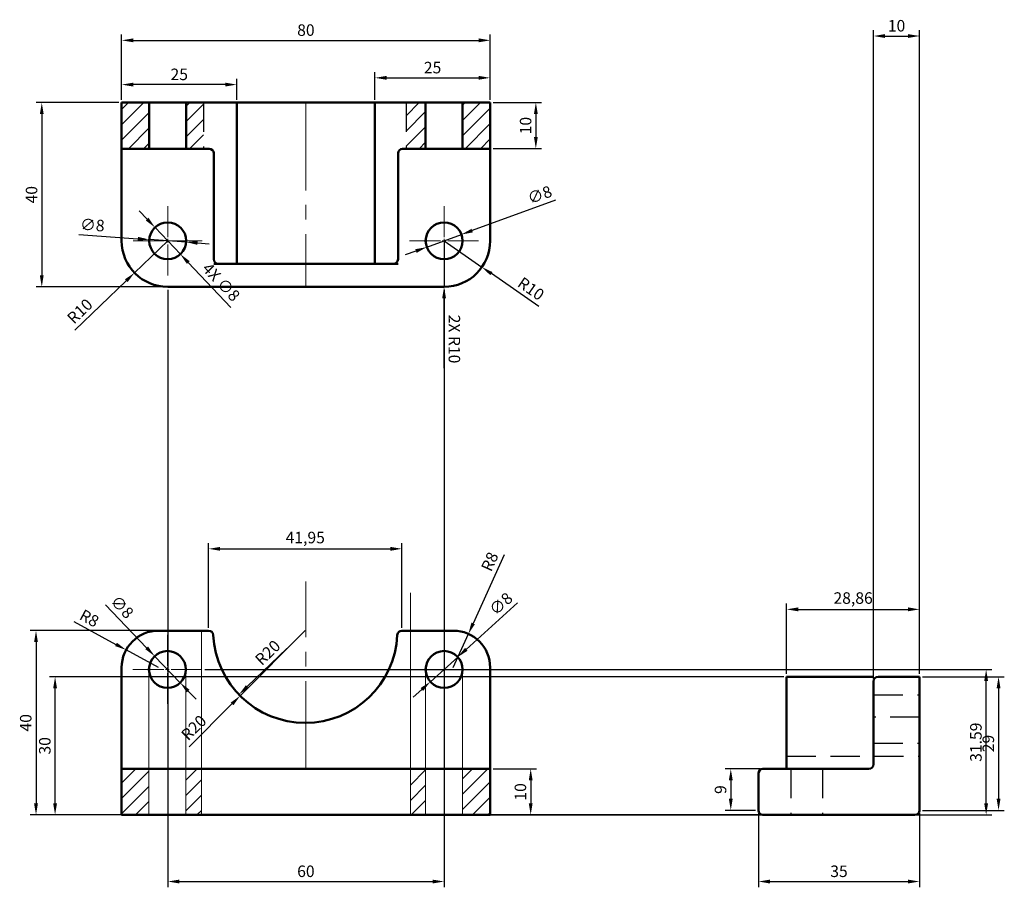
# Model space of a CAD drawing. Units: millimetres. Extents: x 1831 to 2045, y 920 to 1109.
import ezdxf

# ---------------------------------------------------------------- set-up
doc = ezdxf.new("R2010")
doc.units = ezdxf.units.MM
doc.linetypes.add('CENTER2', pattern=[28.575, 19.05, -3.175, 3.175, -3.175])
doc.linetypes.add('HIDDEN', pattern=[9.525, 6.35, -3.175])
for name, color, linetype, lineweight in [('M-CNTR', 4, 'CENTER2', 18), ('M-CONS', 8, 'Continuous', 13), ('M-DIMS', 2, 'Continuous', 25), ('M-HATC', 8, 'Continuous', 18), ('M-HIDN', 3, 'HIDDEN', 25), ('M-OUTL', 7, 'Continuous', 50)]:
    doc.layers.add(name, color=color, linetype=linetype, lineweight=lineweight)
doc.styles.get("Standard").update_dxf_attribs({"font": 'arial.ttf'})
doc.dimstyles.new('ISO-25', dxfattribs={"dimtxt": 2.5, "dimasz": 2.5, "dimexe": 1.25, "dimexo": 0.625, "dimtad": 1, "dimtxsty": 'Standard', "dimcen": 2.5, "dimadec": 0, "dimazin": 0, "dimtfac": 1, "dimtmove": 0, "dimatfit": 3, "dimfxl": 1, "dimarcsym": 0})

# ---------------------------------------------------------------- blocks, each defined once
blk = doc.blocks.new('*D1')
at = {"layer": 'Defpoints', "color": 0, "lineweight": 30, "transparency": 16777216}
for p in [(1914.1, 993.68), (1872.14, 975.92), (1914.1, 975.92)]:
    blk.add_point(p, dxfattribs=at)
at = {"layer": 'M-DIMS', "color": 0, "lineweight": -2, "transparency": 16777216}
for p, q in [((1872.14, 976.54), (1872.14, 994.93)), ((1914.1, 976.54), (1914.1, 994.93)), ((1874.64, 993.68), (1911.6, 993.68))]:
    blk.add_line(p, q, dxfattribs=at)
at = {"layer": 'M-DIMS', "color": 0, "lineweight": 30, "transparency": 16777216}
for points in [[(1874.64, 994.09), (1874.64, 993.26), (1872.14, 993.68)], [(1911.6, 994.09), (1911.6, 993.26), (1914.1, 993.68)]]:
    blk.add_solid(points, dxfattribs=at)
at = {"layer": 'M-DIMS', "color": 0, "transparency": 16777216, "insert": (1893.12, 995.8), "char_height": 2.5, "attachment_point": 5}
blk.add_mtext('41,95', dxfattribs=at)
blk = doc.blocks.new('*D2')
at = {"layer": 'Defpoints', "color": 0, "lineweight": 30, "transparency": 16777216}
for p in [(1933.26, 1104.04), (1853.26, 1090.53), (1933.26, 1090.53)]:
    blk.add_point(p, dxfattribs=at)
at = {"layer": 'M-DIMS', "color": 0, "lineweight": -2, "transparency": 16777216}
for p, q in [((1853.26, 1091.15), (1853.26, 1105.29)), ((1933.26, 1091.15), (1933.26, 1105.29)), ((1855.76, 1104.04), (1930.76, 1104.04))]:
    blk.add_line(p, q, dxfattribs=at)
at = {"layer": 'M-DIMS', "color": 0, "lineweight": 30, "transparency": 16777216}
for points in [[(1855.76, 1104.46), (1855.76, 1103.62), (1853.26, 1104.04)], [(1930.76, 1104.46), (1930.76, 1103.62), (1933.26, 1104.04)]]:
    blk.add_solid(points, dxfattribs=at)
at = {"layer": 'M-DIMS', "color": 0, "transparency": 16777216, "insert": (1893.26, 1105.94), "char_height": 2.5, "attachment_point": 5}
blk.add_mtext('80', dxfattribs=at)
blk = doc.blocks.new('*D3')
at = {"layer": 'Defpoints', "color": 0, "lineweight": 30, "transparency": 16777216}
for p in [(1853.26, 1090.53), (1835.92, 1050.53), (1863.26, 1050.53)]:
    blk.add_point(p, dxfattribs=at)
at = {"layer": 'M-DIMS', "color": 0, "lineweight": -2, "transparency": 16777216}
for p, q in [((1852.63, 1090.53), (1834.67, 1090.53)), ((1835.92, 1088.03), (1835.92, 1053.03)), ((1862.63, 1050.53), (1834.67, 1050.53))]:
    blk.add_line(p, q, dxfattribs=at)
at = {"layer": 'M-DIMS', "color": 0, "lineweight": 30, "transparency": 16777216}
for points in [[(1835.5, 1088.03), (1836.33, 1088.03), (1835.92, 1090.53)], [(1835.5, 1053.03), (1836.33, 1053.03), (1835.92, 1050.53)]]:
    blk.add_solid(points, dxfattribs=at)
at = {"layer": 'M-DIMS', "color": 0, "transparency": 16777216, "insert": (1834.02, 1070.53), "char_height": 2.5, "attachment_point": 5, "rotation": 90}
blk.add_mtext('40', dxfattribs=at)
blk = doc.blocks.new('*U4')
at = {"layer": 'M-CNTR', "color": 0, "transparency": 16777216}
for p, q in [((0, 0.8), (0, 7.5)), ((-7.5, 0), (-0.8, 0)), ((0.8, 0), (7.5, 0)), ((0, -7.5), (0, -0.8))]:
    blk.add_line(p, q, dxfattribs=at)
at = {"layer": 'M-CNTR', "color": 0, "linetype": 'Continuous', "transparency": 16777216}
for p, q in [((-0.4, 0), (0.4, 0)), ((0, -0.4), (0, 0.4))]:
    blk.add_line(p, q, dxfattribs=at)
blk = doc.blocks.new('*U5')
at = {"layer": 'M-CNTR', "color": 0, "transparency": 16777216}
for p, q in [((0, 0.8), (0, 7.5)), ((-7.5, 0), (-0.8, 0)), ((0.8, 0), (7.5, 0)), ((0, -7.5), (0, -0.8))]:
    blk.add_line(p, q, dxfattribs=at)
at = {"layer": 'M-CNTR', "color": 0, "linetype": 'Continuous', "transparency": 16777216}
for p, q in [((-0.4, 0), (0.4, 0)), ((0, -0.4), (0, 0.4))]:
    blk.add_line(p, q, dxfattribs=at)
blk = doc.blocks.new('*U6')
at = {"layer": 'M-CNTR', "color": 0, "transparency": 16777216}
for p, q in [((0, 0.8), (0, 7.5)), ((-7.5, 0), (-0.8, 0)), ((0.8, 0), (7.5, 0)), ((0, -7.5), (0, -0.8))]:
    blk.add_line(p, q, dxfattribs=at)
at = {"layer": 'M-CNTR', "color": 0, "linetype": 'Continuous', "transparency": 16777216}
for p, q in [((-0.4, 0), (0.4, 0)), ((0, -0.4), (0, 0.4))]:
    blk.add_line(p, q, dxfattribs=at)
blk = doc.blocks.new('*U7')
at = {"layer": 'M-CNTR', "color": 0, "transparency": 16777216}
for p, q in [((0, 0.8), (0, 7.5)), ((-7.5, 0), (-0.8, 0)), ((0.8, 0), (7.5, 0)), ((0, -7.5), (0, -0.8))]:
    blk.add_line(p, q, dxfattribs=at)
at = {"layer": 'M-CNTR', "color": 0, "linetype": 'Continuous', "transparency": 16777216}
for p, q in [((-0.4, 0), (0.4, 0)), ((0, -0.4), (0, 0.4))]:
    blk.add_line(p, q, dxfattribs=at)
blk = doc.blocks.new('*D8')
at = {"layer": 'Defpoints', "color": 0, "lineweight": 30, "transparency": 16777216}
for p in [(1893.12, 975.92), (1878.71, 962.04)]:
    blk.add_point(p, dxfattribs=at)
at = {"layer": 'M-DIMS', "color": 0, "lineweight": -2, "transparency": 16777216}
blk.add_line((1889.11, 972.05), (1880.51, 963.78), dxfattribs=at)
at = {"layer": 'M-DIMS', "color": 0, "lineweight": 30, "transparency": 16777216}
blk.add_solid([(1880.23, 964.08), (1880.8, 963.48), (1878.71, 962.04)], dxfattribs=at)
at = {"layer": 'M-DIMS', "color": 0, "transparency": 16777216, "insert": (1885.19, 970.92), "char_height": 2.5, "attachment_point": 5, "rotation": 43.9159}
blk.add_mtext('R20', dxfattribs=at)
blk = doc.blocks.new('*D9')
at = {"layer": 'Defpoints', "color": 0, "lineweight": 30, "transparency": 16777216}
for p in [(1926.22, 970.19), (1920.29, 964.83)]:
    blk.add_point(p, dxfattribs=at)
at = {"layer": 'M-DIMS', "color": 0, "lineweight": -2, "transparency": 16777216}
for p, q in [((1939.21, 981.92), (1928.08, 971.86)), ((1920.29, 964.83), (1926.22, 970.19)), ((1918.43, 963.15), (1916.58, 961.48))]:
    blk.add_line(p, q, dxfattribs=at)
at = {"layer": 'M-DIMS', "color": 0, "lineweight": 30, "transparency": 16777216}
for points in [[(1927.8, 972.17), (1928.36, 971.56), (1926.22, 970.19)], [(1918.15, 963.46), (1918.71, 962.84), (1920.29, 964.83)]]:
    blk.add_solid(points, dxfattribs=at)
at = {"layer": 'M-DIMS', "color": 0, "transparency": 16777216, "insert": (1935.81, 981.5), "char_height": 2.5, "attachment_point": 5, "rotation": 42.0862}
blk.add_mtext('∅8', dxfattribs=at)
blk = doc.blocks.new('*D10')
at = {"layer": 'Defpoints', "color": 0, "lineweight": 30, "transparency": 16777216}
for p in [(1860.42, 970.39), (1865.96, 964.62)]:
    blk.add_point(p, dxfattribs=at)
at = {"layer": 'M-DIMS', "color": 0, "lineweight": -2, "transparency": 16777216}
for p, q in [((1849.76, 981.49), (1858.69, 972.2)), ((1865.96, 964.62), (1860.42, 970.39)), ((1867.69, 962.82), (1869.42, 961.02))]:
    blk.add_line(p, q, dxfattribs=at)
at = {"layer": 'M-DIMS', "color": 0, "lineweight": 30, "transparency": 16777216}
for points in [[(1858.99, 972.49), (1858.39, 971.91), (1860.42, 970.39)], [(1867.99, 963.11), (1867.39, 962.53), (1865.96, 964.62)]]:
    blk.add_solid(points, dxfattribs=at)
at = {"layer": 'M-DIMS', "color": 0, "transparency": 16777216, "insert": (1853.13, 980.83), "char_height": 2.5, "attachment_point": 5, "rotation": 313.8374}
blk.add_mtext('∅8', dxfattribs=at)
blk = doc.blocks.new('*D11')
at = {"layer": 'Defpoints', "color": 0, "lineweight": 30, "transparency": 16777216}
for p in [(1927.01, 1061.89), (1919.5, 1059.16)]:
    blk.add_point(p, dxfattribs=at)
at = {"layer": 'M-DIMS', "color": 0, "lineweight": -2, "transparency": 16777216}
for p, q in [((1947.43, 1069.32), (1929.36, 1062.75)), ((1919.5, 1059.16), (1927.01, 1061.89)), ((1917.15, 1058.31), (1914.8, 1057.45))]:
    blk.add_line(p, q, dxfattribs=at)
at = {"layer": 'M-DIMS', "color": 0, "lineweight": 30, "transparency": 16777216}
for points in [[(1929.22, 1063.14), (1929.51, 1062.36), (1927.01, 1061.89)], [(1917, 1058.7), (1917.29, 1057.91), (1919.5, 1059.16)]]:
    blk.add_solid(points, dxfattribs=at)
at = {"layer": 'M-DIMS', "color": 0, "transparency": 16777216, "insert": (1944.12, 1070.21), "char_height": 2.5, "attachment_point": 5, "rotation": 19.9841}
blk.add_mtext('∅8', dxfattribs=at)
blk = doc.blocks.new('*D12')
at = {"layer": 'Defpoints', "color": 0, "lineweight": 30, "transparency": 16777216}
for p in [(1859.27, 1060.8), (1867.25, 1060.25)]:
    blk.add_point(p, dxfattribs=at)
at = {"layer": 'M-DIMS', "color": 0, "lineweight": -2, "transparency": 16777216}
for p, q in [((1843.94, 1061.87), (1856.77, 1060.98)), ((1867.25, 1060.25), (1859.27, 1060.8)), ((1869.74, 1060.08), (1872.23, 1059.9))]:
    blk.add_line(p, q, dxfattribs=at)
at = {"layer": 'M-DIMS', "color": 0, "lineweight": 30, "transparency": 16777216}
for points in [[(1856.8, 1061.39), (1856.74, 1060.56), (1859.27, 1060.8)], [(1869.77, 1060.49), (1869.71, 1059.66), (1867.25, 1060.25)]]:
    blk.add_solid(points, dxfattribs=at)
at = {"layer": 'M-DIMS', "color": 0, "transparency": 16777216, "insert": (1846.88, 1063.64), "char_height": 2.5, "attachment_point": 5, "rotation": 356.0256}
blk.add_mtext('∅8', dxfattribs=at)
blk = doc.blocks.new('*D13')
at = {"layer": 'Defpoints', "color": 0, "lineweight": 30, "transparency": 16777216}
for p in [(1923.26, 1060.53), (1931.47, 1054.82)]:
    blk.add_point(p, dxfattribs=at)
at = {"layer": 'M-DIMS', "color": 0, "lineweight": -2, "transparency": 16777216}
for p, q in [((1923.26, 1060.53), (1931.47, 1054.82)), ((1943.83, 1046.24), (1933.52, 1053.4))]:
    blk.add_line(p, q, dxfattribs=at)
at = {"layer": 'M-DIMS', "color": 0, "lineweight": 30, "transparency": 16777216}
blk.add_solid([(1933.76, 1053.74), (1933.29, 1053.06), (1931.47, 1054.82)], dxfattribs=at)
at = {"layer": 'M-DIMS', "color": 0, "transparency": 16777216, "insert": (1941.95, 1049.86), "char_height": 2.5, "attachment_point": 5, "rotation": 325.2351}
blk.add_mtext('R10', dxfattribs=at)
blk = doc.blocks.new('*D14')
at = {"layer": 'Defpoints', "color": 0, "lineweight": 30, "transparency": 16777216}
for p in [(1863.26, 1060.53), (1856.05, 1053.59)]:
    blk.add_point(p, dxfattribs=at)
at = {"layer": 'M-DIMS', "color": 0, "lineweight": -2, "transparency": 16777216}
for p, q in [((1863.26, 1060.53), (1856.05, 1053.59)), ((1843.13, 1041.15), (1854.25, 1051.86))]:
    blk.add_line(p, q, dxfattribs=at)
at = {"layer": 'M-DIMS', "color": 0, "lineweight": 30, "transparency": 16777216}
blk.add_solid([(1853.96, 1052.16), (1854.54, 1051.56), (1856.05, 1053.59)], dxfattribs=at)
at = {"layer": 'M-DIMS', "color": 0, "transparency": 16777216, "insert": (1844.41, 1045.02), "char_height": 2.5, "attachment_point": 5, "rotation": 43.9113}
blk.add_mtext('R10', dxfattribs=at)
blk = doc.blocks.new('*D15')
at = {"layer": 'Defpoints', "color": 0, "lineweight": 30, "transparency": 16777216}
for p in [(1928.54, 975.21), (1925.26, 967.92)]:
    blk.add_point(p, dxfattribs=at)
at = {"layer": 'M-DIMS', "color": 0, "lineweight": -2, "transparency": 16777216}
for p, q in [((1936.28, 992.4), (1929.57, 977.49)), ((1925.26, 967.92), (1928.54, 975.21))]:
    blk.add_line(p, q, dxfattribs=at)
at = {"layer": 'M-DIMS', "color": 0, "lineweight": 30, "transparency": 16777216}
blk.add_solid([(1929.19, 977.66), (1929.95, 977.32), (1928.54, 975.21)], dxfattribs=at)
at = {"layer": 'M-DIMS', "color": 0, "transparency": 16777216, "insert": (1933.46, 990.77), "char_height": 2.5, "attachment_point": 5, "rotation": 65.7651}
blk.add_mtext('R8', dxfattribs=at)
blk = doc.blocks.new('*D16')
at = {"layer": 'Defpoints', "color": 0, "lineweight": 30, "transparency": 16777216}
for p in [(1854.23, 971.74), (1861.26, 967.92)]:
    blk.add_point(p, dxfattribs=at)
at = {"layer": 'M-DIMS', "color": 0, "lineweight": -2, "transparency": 16777216}
for p, q in [((1842.86, 977.93), (1852.03, 972.93)), ((1861.26, 967.92), (1854.23, 971.74))]:
    blk.add_line(p, q, dxfattribs=at)
at = {"layer": 'M-DIMS', "color": 0, "lineweight": 30, "transparency": 16777216}
blk.add_solid([(1852.23, 973.3), (1851.83, 972.57), (1854.23, 971.74)], dxfattribs=at)
at = {"layer": 'M-DIMS', "color": 0, "transparency": 16777216, "insert": (1846.09, 978.33), "char_height": 2.5, "attachment_point": 5, "rotation": 331.4476}
blk.add_mtext('R8', dxfattribs=at)
blk = doc.blocks.new('*D17')
at = {"layer": 'Defpoints', "color": 0, "lineweight": 30, "transparency": 16777216}
for p in [(1933.26, 945.92), (1933.26, 935.92), (1942.06, 935.92)]:
    blk.add_point(p, dxfattribs=at)
at = {"layer": 'M-DIMS', "color": 0, "lineweight": -2, "transparency": 16777216}
for p, q in [((1933.88, 945.92), (1943.31, 945.92)), ((1942.06, 943.42), (1942.06, 938.42)), ((1933.88, 935.92), (1943.31, 935.92))]:
    blk.add_line(p, q, dxfattribs=at)
at = {"layer": 'M-DIMS', "color": 0, "lineweight": 30, "transparency": 16777216}
for points in [[(1941.65, 943.42), (1942.48, 943.42), (1942.06, 945.92)], [(1941.65, 938.42), (1942.48, 938.42), (1942.06, 935.92)]]:
    blk.add_solid(points, dxfattribs=at)
at = {"layer": 'M-DIMS', "color": 0, "transparency": 16777216, "insert": (1940.16, 940.92), "char_height": 2.5, "attachment_point": 5, "rotation": 90}
blk.add_mtext('10', dxfattribs=at)
blk = doc.blocks.new('*D18')
at = {"layer": 'Defpoints', "color": 0, "lineweight": 30, "transparency": 16777216}
for p in [(1861.26, 975.92), (1834.67, 935.92), (1853.26, 935.92)]:
    blk.add_point(p, dxfattribs=at)
at = {"layer": 'M-DIMS', "color": 0, "lineweight": -2, "transparency": 16777216}
for p, q in [((1860.63, 975.92), (1833.42, 975.92)), ((1834.67, 973.42), (1834.67, 938.42)), ((1852.63, 935.92), (1833.42, 935.92))]:
    blk.add_line(p, q, dxfattribs=at)
at = {"layer": 'M-DIMS', "color": 0, "lineweight": 30, "transparency": 16777216}
for points in [[(1834.25, 973.42), (1835.08, 973.42), (1834.67, 975.92)], [(1834.25, 938.42), (1835.08, 938.42), (1834.67, 935.92)]]:
    blk.add_solid(points, dxfattribs=at)
at = {"layer": 'M-DIMS', "color": 0, "transparency": 16777216, "insert": (1832.76, 955.92), "char_height": 2.5, "attachment_point": 5, "rotation": 90}
blk.add_mtext('40', dxfattribs=at)
blk = doc.blocks.new('*D19')
at = {"layer": 'Defpoints', "color": 0, "lineweight": 30, "transparency": 16777216}
for p in [(2026.49, 980.54), (1997.63, 965.92), (2026.49, 965.92)]:
    blk.add_point(p, dxfattribs=at)
at = {"layer": 'M-DIMS', "color": 0, "lineweight": -2, "transparency": 16777216}
for p, q in [((1997.63, 966.54), (1997.63, 981.79)), ((2026.49, 966.54), (2026.49, 981.79)), ((2000.13, 980.54), (2023.99, 980.54))]:
    blk.add_line(p, q, dxfattribs=at)
at = {"layer": 'M-DIMS', "color": 0, "lineweight": 30, "transparency": 16777216}
for points in [[(2000.13, 980.96), (2000.13, 980.12), (1997.63, 980.54)], [(2023.99, 980.96), (2023.99, 980.12), (2026.49, 980.54)]]:
    blk.add_solid(points, dxfattribs=at)
at = {"layer": 'M-DIMS', "color": 0, "transparency": 16777216, "insert": (2012.06, 982.67), "char_height": 2.5, "attachment_point": 5}
blk.add_mtext('28,86', dxfattribs=at)
blk = doc.blocks.new('*D20')
at = {"layer": 'Defpoints', "color": 0, "lineweight": 30, "transparency": 16777216}
for p in [(1992.49, 945.92), (1985.5, 936.92), (1991.49, 936.92)]:
    blk.add_point(p, dxfattribs=at)
at = {"layer": 'M-DIMS', "color": 0, "lineweight": -2, "transparency": 16777216}
for p, q in [((1991.86, 945.92), (1984.25, 945.92)), ((1985.5, 943.42), (1985.5, 939.42)), ((1990.86, 936.92), (1984.25, 936.92))]:
    blk.add_line(p, q, dxfattribs=at)
at = {"layer": 'M-DIMS', "color": 0, "lineweight": 30, "transparency": 16777216}
for points in [[(1985.08, 943.42), (1985.92, 943.42), (1985.5, 945.92)], [(1985.08, 939.42), (1985.92, 939.42), (1985.5, 936.92)]]:
    blk.add_solid(points, dxfattribs=at)
at = {"layer": 'M-DIMS', "color": 0, "transparency": 16777216, "insert": (1983.6, 941.42), "char_height": 2.5, "attachment_point": 5, "rotation": 90}
blk.add_mtext('9', dxfattribs=at)
blk = doc.blocks.new('*D21')
at = {"layer": 'Defpoints', "color": 0, "lineweight": 30, "transparency": 16777216}
for p in [(1933.26, 1090.53), (1933.26, 1080.53), (1943.18, 1080.53)]:
    blk.add_point(p, dxfattribs=at)
at = {"layer": 'M-DIMS', "color": 0, "lineweight": -2, "transparency": 16777216}
for p, q in [((1933.88, 1090.53), (1944.43, 1090.53)), ((1943.18, 1088.03), (1943.18, 1083.03)), ((1933.88, 1080.53), (1944.43, 1080.53))]:
    blk.add_line(p, q, dxfattribs=at)
at = {"layer": 'M-DIMS', "color": 0, "lineweight": 30, "transparency": 16777216}
for points in [[(1942.77, 1088.03), (1943.6, 1088.03), (1943.18, 1090.53)], [(1942.77, 1083.03), (1943.6, 1083.03), (1943.18, 1080.53)]]:
    blk.add_solid(points, dxfattribs=at)
at = {"layer": 'M-DIMS', "color": 0, "transparency": 16777216, "insert": (1941.28, 1085.53), "char_height": 2.5, "attachment_point": 5, "rotation": 90}
blk.add_mtext('10', dxfattribs=at)
blk = doc.blocks.new('*D22')
at = {"layer": 'Defpoints', "color": 0, "lineweight": 30, "transparency": 16777216}
for p in [(2026.49, 965.92), (2026.49, 936.92), (2043.63, 936.92)]:
    blk.add_point(p, dxfattribs=at)
at = {"layer": 'M-DIMS', "color": 0, "lineweight": -2, "transparency": 16777216}
for p, q in [((2027.11, 965.92), (2044.88, 965.92)), ((2043.63, 963.42), (2043.63, 939.42)), ((2027.11, 936.92), (2044.88, 936.92))]:
    blk.add_line(p, q, dxfattribs=at)
at = {"layer": 'M-DIMS', "color": 0, "lineweight": 30, "transparency": 16777216}
for points in [[(2043.22, 963.42), (2044.05, 963.42), (2043.63, 965.92)], [(2043.22, 939.42), (2044.05, 939.42), (2043.63, 936.92)]]:
    blk.add_solid(points, dxfattribs=at)
at = {"layer": 'M-DIMS', "color": 0, "transparency": 16777216, "insert": (2041.73, 951.42), "char_height": 2.5, "attachment_point": 5, "rotation": 90}
blk.add_mtext('29', dxfattribs=at)
blk = doc.blocks.new('*D23')
at = {"layer": 'Defpoints', "color": 0, "lineweight": 30, "transparency": 16777216}
for p in [(1933.26, 1095.9), (1908.26, 1090.53), (1933.26, 1090.53)]:
    blk.add_point(p, dxfattribs=at)
at = {"layer": 'M-DIMS', "color": 0, "lineweight": -2, "transparency": 16777216}
for p, q in [((1908.26, 1091.15), (1908.26, 1097.15)), ((1933.26, 1091.15), (1933.26, 1097.15)), ((1910.76, 1095.9), (1930.76, 1095.9))]:
    blk.add_line(p, q, dxfattribs=at)
at = {"layer": 'M-DIMS', "color": 0, "lineweight": 30, "transparency": 16777216}
for points in [[(1910.76, 1096.32), (1910.76, 1095.49), (1908.26, 1095.9)], [(1930.76, 1096.32), (1930.76, 1095.49), (1933.26, 1095.9)]]:
    blk.add_solid(points, dxfattribs=at)
at = {"layer": 'M-DIMS', "color": 0, "transparency": 16777216, "insert": (1920.76, 1097.8), "char_height": 2.5, "attachment_point": 5}
blk.add_mtext('25', dxfattribs=at)
blk = doc.blocks.new('*D24')
at = {"layer": 'Defpoints', "color": 0, "lineweight": 30, "transparency": 16777216}
for p in [(1853.26, 1094.43), (1853.26, 1090.53), (1878.26, 1090.53)]:
    blk.add_point(p, dxfattribs=at)
at = {"layer": 'M-DIMS', "color": 0, "lineweight": -2, "transparency": 16777216}
for p, q in [((1853.26, 1091.15), (1853.26, 1095.68)), ((1878.26, 1091.15), (1878.26, 1095.68)), ((1875.76, 1094.43), (1855.76, 1094.43))]:
    blk.add_line(p, q, dxfattribs=at)
at = {"layer": 'M-DIMS', "color": 0, "lineweight": 30, "transparency": 16777216}
for points in [[(1855.76, 1094.85), (1855.76, 1094.02), (1853.26, 1094.43)], [(1875.76, 1094.85), (1875.76, 1094.02), (1878.26, 1094.43)]]:
    blk.add_solid(points, dxfattribs=at)
at = {"layer": 'M-DIMS', "color": 0, "transparency": 16777216, "insert": (1865.76, 1096.33), "char_height": 2.5, "attachment_point": 5}
blk.add_mtext('25', dxfattribs=at)
blk = doc.blocks.new('*D25')
at = {"layer": 'Defpoints', "color": 0, "lineweight": 30, "transparency": 16777216}
for p in [(1863.26, 1050.53), (1923.26, 1050.53), (1923.26, 921.47)]:
    blk.add_point(p, dxfattribs=at)
at = {"layer": 'M-DIMS', "color": 0, "lineweight": -2, "transparency": 16777216}
for p, q in [((1863.26, 1049.9), (1863.26, 920.22)), ((1923.26, 1049.9), (1923.26, 920.22)), ((1865.76, 921.47), (1920.76, 921.47))]:
    blk.add_line(p, q, dxfattribs=at)
at = {"layer": 'M-DIMS', "color": 0, "lineweight": 30, "transparency": 16777216}
for points in [[(1865.76, 921.88), (1865.76, 921.05), (1863.26, 921.47)], [(1920.76, 921.88), (1920.76, 921.05), (1923.26, 921.47)]]:
    blk.add_solid(points, dxfattribs=at)
at = {"layer": 'M-DIMS', "color": 0, "transparency": 16777216, "insert": (1893.26, 923.37), "char_height": 2.5, "attachment_point": 5}
blk.add_mtext('60', dxfattribs=at)
blk = doc.blocks.new('*D26')
at = {"layer": 'Defpoints', "color": 0, "lineweight": 30, "transparency": 16777216}
for p in [(1870.69, 967.51), (2040.94, 967.51), (1870.58, 935.92)]:
    blk.add_point(p, dxfattribs=at)
at = {"layer": 'M-DIMS', "color": 0, "lineweight": -2, "transparency": 16777216}
for p, q in [((1871.31, 967.51), (2042.19, 967.51)), ((2040.94, 938.42), (2040.94, 965.01)), ((1871.2, 935.92), (2042.19, 935.92))]:
    blk.add_line(p, q, dxfattribs=at)
at = {"layer": 'M-DIMS', "color": 0, "lineweight": 30, "transparency": 16777216}
for points in [[(2040.52, 965.01), (2041.35, 965.01), (2040.94, 967.51)], [(2040.52, 938.42), (2041.35, 938.42), (2040.94, 935.92)]]:
    blk.add_solid(points, dxfattribs=at)
at = {"layer": 'M-DIMS', "color": 0, "transparency": 16777216, "insert": (2039.04, 951.71), "char_height": 2.5, "attachment_point": 5, "rotation": 90}
blk.add_mtext('31.59', dxfattribs=at)
blk = doc.blocks.new('*D27')
at = {"layer": 'Defpoints', "color": 0, "lineweight": 30, "transparency": 16777216}
for p in [(1991.49, 936.92), (2026.49, 936.92), (2026.49, 921.47)]:
    blk.add_point(p, dxfattribs=at)
at = {"layer": 'M-DIMS', "color": 0, "lineweight": -2, "transparency": 16777216}
for p, q in [((1991.49, 936.29), (1991.49, 920.22)), ((2026.49, 936.29), (2026.49, 920.22)), ((1993.99, 921.47), (2023.99, 921.47))]:
    blk.add_line(p, q, dxfattribs=at)
at = {"layer": 'M-DIMS', "color": 0, "lineweight": 30, "transparency": 16777216}
for points in [[(1993.99, 921.88), (1993.99, 921.05), (1991.49, 921.47)], [(2023.99, 921.88), (2023.99, 921.05), (2026.49, 921.47)]]:
    blk.add_solid(points, dxfattribs=at)
at = {"layer": 'M-DIMS', "color": 0, "transparency": 16777216, "insert": (2008.99, 923.37), "char_height": 2.5, "attachment_point": 5}
blk.add_mtext('35', dxfattribs=at)
blk = doc.blocks.new('*D28')
at = {"layer": 'Defpoints', "color": 0, "lineweight": 30, "transparency": 16777216}
for p in [(1838.81, 965.92), (1997.63, 965.92), (1992.49, 935.92)]:
    blk.add_point(p, dxfattribs=at)
at = {"layer": 'M-DIMS', "color": 0, "lineweight": -2, "transparency": 16777216}
for p, q in [((1997.01, 965.92), (1837.56, 965.92)), ((1838.81, 938.42), (1838.81, 963.42)), ((1991.86, 935.92), (1837.56, 935.92))]:
    blk.add_line(p, q, dxfattribs=at)
at = {"layer": 'M-DIMS', "color": 0, "lineweight": 30, "transparency": 16777216}
for points in [[(1838.39, 963.42), (1839.22, 963.42), (1838.81, 965.92)], [(1838.39, 938.42), (1839.22, 938.42), (1838.81, 935.92)]]:
    blk.add_solid(points, dxfattribs=at)
at = {"layer": 'M-DIMS', "color": 0, "transparency": 16777216, "insert": (1836.9, 950.92), "char_height": 2.5, "attachment_point": 5, "rotation": 90}
blk.add_mtext('30', dxfattribs=at)
blk = doc.blocks.new('*D29')
at = {"layer": 'Defpoints', "color": 0, "lineweight": 30, "transparency": 16777216}
for p in [(2026.49, 1104.98), (2016.49, 964.92), (2026.49, 965.92)]:
    blk.add_point(p, dxfattribs=at)
at = {"layer": 'M-DIMS', "color": 0, "lineweight": -2, "transparency": 16777216}
for p, q in [((2016.49, 965.54), (2016.49, 1106.23)), ((2026.49, 966.54), (2026.49, 1106.23)), ((2018.99, 1104.98), (2023.99, 1104.98))]:
    blk.add_line(p, q, dxfattribs=at)
at = {"layer": 'M-DIMS', "color": 0, "lineweight": 30, "transparency": 16777216}
for points in [[(2018.99, 1105.39), (2018.99, 1104.56), (2016.49, 1104.98)], [(2023.99, 1105.39), (2023.99, 1104.56), (2026.49, 1104.98)]]:
    blk.add_solid(points, dxfattribs=at)
at = {"layer": 'M-DIMS', "color": 0, "transparency": 16777216, "insert": (2021.49, 1106.88), "char_height": 2.5, "attachment_point": 5}
blk.add_mtext('10', dxfattribs=at)
blk = doc.blocks.new('*D30')
at = {"layer": 'Defpoints', "color": 0, "lineweight": 30, "transparency": 16777216}
for p in [(1893.12, 975.92), (1878.98, 961.77)]:
    blk.add_point(p, dxfattribs=at)
at = {"layer": 'M-DIMS', "color": 0, "lineweight": -2, "transparency": 16777216}
for p, q in [((1893.12, 975.92), (1878.98, 961.77)), ((1867.95, 950.73), (1877.21, 960))]:
    blk.add_line(p, q, dxfattribs=at)
at = {"layer": 'M-DIMS', "color": 0, "lineweight": 30, "transparency": 16777216}
blk.add_solid([(1876.92, 960.3), (1877.51, 959.71), (1878.98, 961.77)], dxfattribs=at)
at = {"layer": 'M-DIMS', "color": 0, "transparency": 16777216, "insert": (1869.15, 954.63), "char_height": 2.5, "attachment_point": 5, "rotation": 45.0097}
blk.add_mtext('R20', dxfattribs=at)
blk = doc.blocks.new('*D31')
at = {"layer": 'Defpoints', "color": 0, "lineweight": 30, "transparency": 16777216}
for p in [(1860.5, 1063.43), (1866.01, 1057.62)]:
    blk.add_point(p, dxfattribs=at)
at = {"layer": 'M-DIMS', "color": 0, "lineweight": -2, "transparency": 16777216}
for p, q in [((1858.78, 1065.25), (1857.06, 1067.06)), ((1860.5, 1063.43), (1866.01, 1057.62)), ((1876.98, 1046.04), (1867.73, 1055.81))]:
    blk.add_line(p, q, dxfattribs=at)
at = {"layer": 'M-DIMS', "color": 0, "lineweight": 30, "transparency": 16777216}
for points in [[(1859.09, 1065.53), (1858.48, 1064.96), (1860.5, 1063.43)], [(1868.03, 1056.1), (1867.42, 1055.52), (1866.01, 1057.62)]]:
    blk.add_solid(points, dxfattribs=at)
at = {"layer": 'M-DIMS', "color": 0, "transparency": 16777216, "insert": (1874.64, 1051.37), "char_height": 2.5, "attachment_point": 5, "rotation": 313.4587}
blk.add_mtext('4X ∅8', dxfattribs=at)
blk = doc.blocks.new('*D32')
at = {"layer": 'Defpoints', "color": 0, "lineweight": 30, "transparency": 16777216}
for p in [(1923.26, 1060.53), (1923.26, 1050.53)]:
    blk.add_point(p, dxfattribs=at)
at = {"layer": 'M-DIMS', "color": 0, "lineweight": -2, "transparency": 16777216}
for p, q in [((1923.26, 1060.53), (1923.26, 1050.53)), ((1923.27, 1032.9), (1923.26, 1048.03))]:
    blk.add_line(p, q, dxfattribs=at)
at = {"layer": 'M-DIMS', "color": 0, "lineweight": 30, "transparency": 16777216}
blk.add_solid([(1923.68, 1048.03), (1922.84, 1048.03), (1923.26, 1050.53)], dxfattribs=at)
at = {"layer": 'M-DIMS', "color": 0, "transparency": 16777216, "insert": (1925.17, 1039.21), "char_height": 2.5, "attachment_point": 5, "rotation": 270.026}
blk.add_mtext('2X R10', dxfattribs=at)

msp = doc.modelspace()

# ---------------------------------------------------------------- hatches: boundary and pattern name
at = {"layer": 'M-HATC'}
h = msp.add_hatch(dxfattribs=at)
h.set_pattern_fill('ANSI31', color=256, scale=0.74)
h.paths.add_polyline_path([(1853.255, 1080.527), (1859.255, 1080.527), (1859.255, 1090.527), (1853.255, 1090.527)])
h.paths.add_polyline_path([(1933.255, 1090.527), (1927.255, 1090.527), (1927.255, 1080.527), (1933.255, 1080.527)])
h = msp.add_hatch(dxfattribs=at)
h.set_pattern_fill('ANSI31', color=256, scale=0.74)
h.paths.add_polyline_path([(1871.033, 1090.527), (1867.255, 1090.527), (1867.255, 1080.527), (1871.033, 1080.527)])
h.paths.add_polyline_path([(1915.033, 1080.527), (1919.255, 1080.527), (1919.255, 1090.527), (1915.033, 1090.527)])
h = msp.add_hatch(dxfattribs=at)
h.set_pattern_fill('ANSI31', color=256, scale=0.74)
h.paths.add_polyline_path([(1859.188, 945.915), (1853.255, 945.915), (1853.255, 935.915), (1859.188, 935.915)])
h.paths.add_polyline_path([(1870.576, 945.915), (1867.188, 945.915), (1867.188, 935.915), (1870.576, 935.915)])
h.paths.add_polyline_path([(1919.255, 945.915), (1915.957, 945.915), (1915.957, 935.915), (1919.255, 935.915)])
h.paths.add_polyline_path([(1933.255, 945.915), (1927.255, 945.915), (1927.255, 935.915), (1933.255, 935.915)])

# ---------------------------------------------------------------- linework, layer by layer
at = {"layer": 'M-CNTR'}
for p, q in [((1893.255, 1090.527), (1893.255, 1050.527)), ((1893.255, 945.915), (1893.255, 986.602))]:
    msp.add_line(p, q, dxfattribs=at)
at = {"layer": 'M-CONS'}
for p, q in [((1915.957, 984.137), (1915.957, 935.915)), ((1870.576, 975.915), (1870.576, 935.915)), ((1859.188, 967.508), (1859.188, 935.915)), ((1867.188, 967.508), (1867.188, 935.915)), ((1919.255, 967.508), (1919.255, 935.915)), ((1927.255, 967.508), (1927.255, 935.915))]:
    msp.add_line(p, q, dxfattribs=at)
at = {"layer": 'M-HIDN'}
for p, q in [((1871.033, 1090.527), (1871.033, 1080.527)), ((1915.033, 1090.527), (1915.033, 1080.527)), ((2016.488, 962.021), (2026.488, 962.021)), ((2026.488, 957.114), (2016.488, 957.114)), ((2016.488, 951.518), (2026.488, 951.518)), ((1997.63, 948.678), (2026.488, 948.678)), ((1998.552, 945.915), (1998.552, 935.915)), ((2005.433, 945.915), (2005.433, 935.915))]:
    msp.add_line(p, q, dxfattribs=at)
at = {"layer": 'M-OUTL'}
for p, q in [((1853.255, 1090.527), (1933.255, 1090.527)), ((1853.255, 1090.527), (1853.255, 1060.527)), ((1853.255, 1090.527), (1853.255, 1080.527)), ((1859.255, 1080.527), (1859.255, 1090.527)), ((1867.255, 1080.527), (1867.255, 1090.527)), ((1878.255, 1055.527), (1878.255, 1090.527)), ((1908.255, 1055.527), (1908.255, 1090.527)), ((1919.255, 1080.527), (1919.255, 1090.527)), ((1927.255, 1080.527), (1927.255, 1090.527)), ((1933.255, 1060.527), (1933.255, 1090.527)), ((1853.255, 1080.527), (1872.255, 1080.527)), ((1873.255, 1079.527), (1873.255, 1056.527)), ((1913.255, 1056.527), (1913.255, 1079.527)), ((1914.255, 1080.527), (1933.255, 1080.527)), ((1873.255, 1055.527), (1913.255, 1055.527)), ((1874.255, 1055.527), (1878.255, 1055.527)), ((1912.255, 1055.527), (1908.255, 1055.527)), ((1863.255, 1050.527), (1923.255, 1050.527)), ((1861.255, 975.915), (1872.144, 975.915)), ((1925.255, 975.915), (1914.097, 975.915)), ((1914.097, 975.915), (1923.255, 975.915)), ((1853.255, 945.915), (1853.255, 967.915)), ((1933.255, 945.915), (1933.255, 967.915)), ((2016.488, 965.915), (1997.63, 965.915)), ((1997.63, 965.915), (1997.63, 945.915)), ((2016.488, 964.915), (2016.488, 946.915)), ((2026.488, 965.915), (2017.488, 965.915)), ((2026.488, 936.915), (2026.488, 965.915)), ((1933.255, 945.915), (1853.255, 945.915)), ((1853.255, 945.915), (1853.255, 935.915)), ((1933.255, 935.915), (1933.255, 945.915)), ((1991.488, 936.915), (1991.488, 944.915)), ((1992.488, 945.915), (2015.488, 945.915)), ((1853.255, 935.915), (1933.255, 935.915)), ((1992.488, 935.915), (2025.488, 935.915))]:
    msp.add_line(p, q, dxfattribs=at)
for centre in [(1863.255, 1060.527), (1923.255, 1060.527), (1863.188, 967.508), (1923.255, 967.508)]:
    msp.add_circle(centre, 4, dxfattribs=at)
for centre, radius, start, end in [((1872.255, 1079.527), 1, 0, 90), ((1914.255, 1079.527), 1, 90, 180), ((1863.255, 1060.527), 10, 180, 270), ((1923.255, 1060.527), 10, 270, 0), ((1874.255, 1056.527), 1, 180, 270), ((1912.255, 1056.527), 1, 270, 0), ((1861.255, 967.915), 8, 90, 180), ((1872.144, 974.915), 1, 2.7294, 90), ((1893.12, 975.915), 20, 182.7294, 357.2706), ((1914.097, 974.915), 1, 90, 177.2706), ((1925.255, 967.915), 8, 0, 90), ((2017.488, 964.915), 1, 90, 180), ((1992.488, 944.915), 1, 90, 180), ((2015.488, 946.915), 1, 270, 0), ((1992.488, 936.915), 1, 180, 270), ((2025.488, 936.915), 1, 270, 0)]:
    msp.add_arc(centre, radius, start, end, dxfattribs=at)

# ---------------------------------------------------------------- block references
at = {"layer": 'M-CNTR'}
for name, p in [('*U4', (1863.255, 1060.527)), ('*U5', (1923.255, 1060.527)), ('*U7', (1863.188, 967.508)), ('*U6', (1923.255, 967.508))]:
    msp.add_blockref(name, p, dxfattribs=at)

# ---------------------------------------------------------------- dimensions: what is measured, and where the dimension line sits
at = {"layer": 'M-DIMS'}
for base, p1, p2, override, picture, middle in [((1933.255, 1104.04), (1853.255, 1090.527), (1933.255, 1090.527), {"dimclrd": 0, "dimclre": 0, "dimclrt": 0}, '*D2', (1893.255, 1105.941)), ((2026.488, 1104.977), (2016.488, 964.915), (2026.488, 965.915), {"dimdec": 0, "dimlfac": 1, "dimrnd": 0, "dimzin": 0, "dimdsep": 46, "dimlunit": 2}, '*D29', (2021.488, 1106.878)), ((1933.255, 1095.903), (1908.255, 1090.527), (1933.255, 1090.527), {"dimclrd": 0, "dimclre": 0, "dimclrt": 0}, '*D23', (1920.755, 1097.804)), ((1853.255, 1094.432), (1878.255, 1090.527), (1853.255, 1090.527), {"dimclrd": 0, "dimclre": 0, "dimclrt": 0}, '*D24', (1865.755, 1096.334)), ((1923.255, 921.465), (1863.255, 1050.527), (1923.255, 1050.527), {"dimdec": 0, "dimlfac": 1, "dimrnd": 0, "dimzin": 0, "dimdsep": 46, "dimlunit": 2}, '*D25', (1893.255, 923.367)), ((1914.097, 993.677), (1872.144, 975.915), (1914.097, 975.915), {"dimclrd": 0, "dimclre": 0, "dimclrt": 0}, '*D1', (1893.12, 995.804)), ((2026.488, 980.539), (1997.63, 965.915), (2026.488, 965.915), {"dimclrd": 0, "dimclre": 0, "dimclrt": 0}, '*D19', (2012.059, 982.667)), ((2026.488, 921.465), (1991.488, 936.915), (2026.488, 936.915), {"dimdec": 0, "dimlfac": 1, "dimrnd": 0, "dimzin": 0, "dimdsep": 46, "dimlunit": 2}, '*D27', (2008.988, 923.367))]:
    dim = msp.add_linear_dim(base=base, p1=p1, p2=p2, dimstyle='ISO-25', override=override, dxfattribs=at)
    dim.commit()
    dim.dimension.update_dxf_attribs({"geometry": picture, "text_midpoint": middle})
for base, p1, p2, override, picture, middle in [((1835.918, 1050.527), (1853.255, 1090.527), (1863.255, 1050.527), {"dimclrd": 0, "dimclre": 0, "dimclrt": 0}, '*D3', (1834.017, 1070.527)), ((1943.183, 1080.527), (1933.255, 1090.527), (1933.255, 1080.527), {"dimclrd": 0, "dimclre": 0, "dimclrt": 0}, '*D21', (1941.281, 1085.527)), ((1834.666, 935.915), (1861.255, 975.915), (1853.255, 935.915), {"dimclrd": 0, "dimclre": 0, "dimclrt": 0}, '*D18', (1832.765, 955.915)), ((2040.938, 967.508), (1870.576, 935.915), (1870.688, 967.508), {"dimdec": 2, "dimlfac": 1, "dimrnd": 0, "dimzin": 0, "dimdsep": 46, "dimlunit": 2}, '*D26', (2039.036, 951.712)), ((1838.805, 965.915), (1992.488, 935.915), (1997.63, 965.915), {"dimdec": 0, "dimlfac": 1, "dimrnd": 0, "dimzin": 0, "dimdsep": 46, "dimlunit": 2}, '*D28', (1836.903, 950.915)), ((2043.632, 936.915), (2026.488, 965.915), (2026.488, 936.915), {"dimclrd": 0, "dimclre": 0, "dimclrt": 0}, '*D22', (2041.731, 951.415)), ((1942.063, 935.915), (1933.255, 945.915), (1933.255, 935.915), {"dimclrd": 0, "dimclre": 0, "dimclrt": 0}, '*D17', (1940.161, 940.915)), ((1985.501, 936.915), (1992.488, 945.915), (1991.488, 936.915), {"dimclrd": 0, "dimclre": 0, "dimclrt": 0}, '*D20', (1983.6, 941.415))]:
    dim = msp.add_linear_dim(base=base, p1=p1, p2=p2, angle=90, dimstyle='ISO-25', override=override, dxfattribs=at)
    dim.commit()
    dim.dimension.update_dxf_attribs({"geometry": picture, "text_midpoint": middle})
for p1, p2, picture, middle in [((1919.496, 1059.16), (1927.015, 1061.894), '*D11', (1944.796, 1068.36)), ((1867.246, 1060.25), (1859.265, 1060.804), '*D12', (1846.744, 1061.674)), ((1865.958, 964.623), (1860.417, 970.393), '*D10', (1851.708, 979.464)), ((1920.287, 964.827), (1926.224, 970.189), '*D9', (1937.13, 980.039))]:
    dim = msp.add_diameter_dim_2p(p1=p1, p2=p2, dimstyle='ISO-25', override={"dimclrd": 0, "dimclre": 0, "dimclrt": 0}, dxfattribs=at)
    dim.commit()
    dim.dimension.update_dxf_attribs({"geometry": picture, "text_midpoint": middle, "dimtype": 163})
dim = msp.add_diameter_dim_2p(p1=(1860.504, 1063.43), p2=(1866.007, 1057.623), text='4X <>', dimstyle='ISO-25', override={"dimdec": 0, "dimlfac": 1, "dimrnd": 0, "dimzin": 0, "dimdsep": 46, "dimlunit": 2}, dxfattribs=at)
dim.commit()
dim.dimension.update_dxf_attribs({"geometry": '*D31', "text_midpoint": (1873.213, 1050.019), "dimtype": 163})
for center, mpoint, override, picture, middle in [((1863.255, 1060.527), (1856.051, 1053.591), {"dimclrd": 0, "dimclre": 0, "dimclrt": 0}, '*D14', (1845.725, 1043.651)), ((1923.255, 1060.527), (1931.47, 1054.825), {"dimclrd": 0, "dimclre": 0, "dimclrt": 0}, '*D13', (1940.868, 1048.302)), ((1925.255, 967.915), (1928.539, 975.21), {"dimclrd": 0, "dimclre": 0, "dimclrt": 0}, '*D15', (1935.193, 989.992)), ((1861.255, 967.915), (1854.228, 971.739), {"dimclrd": 0, "dimclre": 0, "dimclrt": 0}, '*D16', (1845.18, 976.663)), ((1893.12, 975.915), (1878.981, 961.771), {"dimdec": 0, "dimlfac": 1, "dimrnd": 0, "dimzin": 0, "dimdsep": 46, "dimlunit": 2}, '*D30', (1870.497, 953.284)), ((1893.12, 975.915), (1878.713, 962.043), {"dimclrd": 0, "dimclre": 0, "dimclrt": 0}, '*D8', (1886.509, 969.55))]:
    dim = msp.add_radius_dim(center=center, mpoint=mpoint, dimstyle='ISO-25', override=override, dxfattribs=at)
    dim.commit()
    dim.dimension.update_dxf_attribs({"geometry": picture, "text_midpoint": middle, "dimtype": 164})
dim = msp.add_radius_dim(center=(1923.255, 1060.527), mpoint=(1923.26, 1050.527), text='2X <>', dimstyle='ISO-25', override={"dimdec": 0, "dimlfac": 1, "dimrnd": 0, "dimzin": 0, "dimdsep": 46, "dimlunit": 2}, dxfattribs=at)
dim.commit()
dim.dimension.update_dxf_attribs({"geometry": '*D32', "text_midpoint": (1925.167, 1039.213)})

doc.saveas('drawing.dxf')
